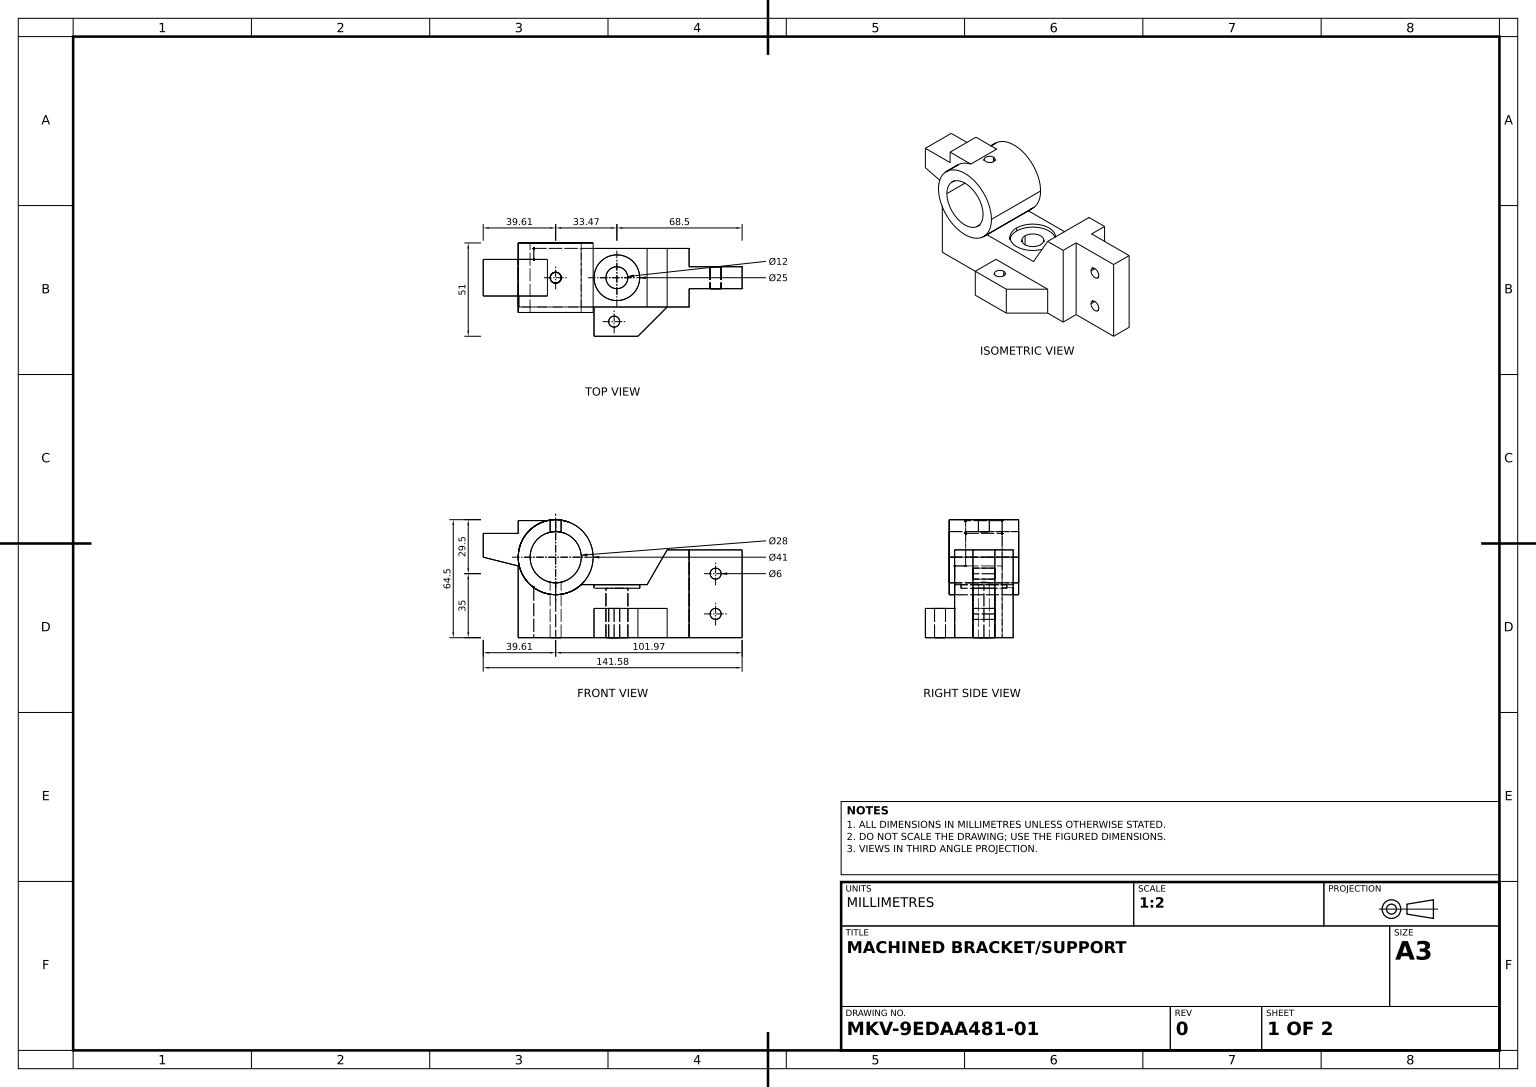
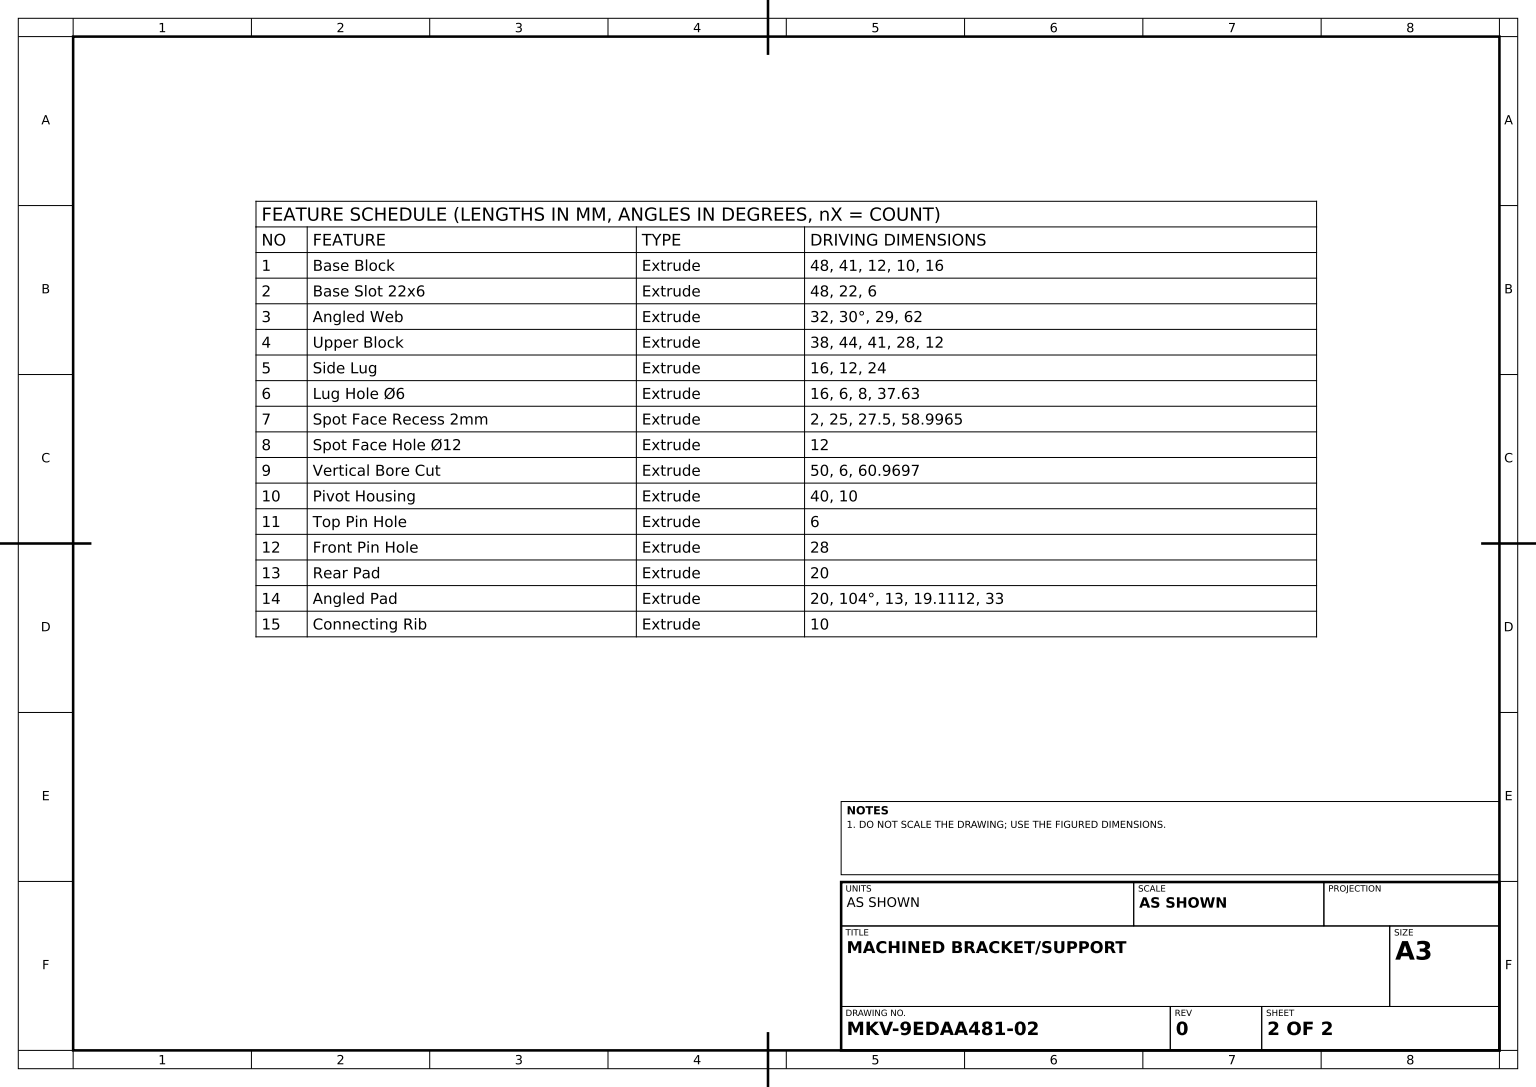
from build123d import *

# Parameters (mm, degrees)
BASE_BLOCK_DEPTH           = 24
BASE_SLOT_SKETCH_R         = 3
BASE_SLOT_22X6_DEPTH       = 48
ANGLED_WEB_DEPTH           = 16
UPPER_BLOCK_SKETCH_R       = 20.5
UPPER_BLOCK_SKETCH_R_2     = 14
UPPER_BLOCK_DEPTH          = 19
SIDE_LUG_SKETCH_W          = 24
SIDE_LUG_SKETCH_H          = 16
SIDE_LUG_DEPTH             = 16
LUG_HOLE_SKETCH_R          = 3
LUG_HOLE_6_DEPTH           = 16
SPOT_FACE_RECESS_SKETCH_R  = 12.5
SPOT_FACE_RECESS_2MM_DEPTH = 2
SPOT_FACE_HOLE_SKETCH_R    = 6
SPOT_FACE_HOLE_12_DEPTH    = 96.223708731
VERTICAL_BORE_SKETCH_R     = 3
VERTICAL_BORE_CUT_DEPTH    = 50
PIVOT_HOUSING_DEPTH        = 40
TOP_PIN_HOLE_DEPTH         = 97.444568168
TOP_PIN_HOLE_DEPTH_BACK    = 97.444568168
TOP_PIN_HOLE_SKETCH_R      = 3
FRONT_PIN_HOLE_DEPTH       = 97.444568168
FRONT_PIN_HOLE_DEPTH_BACK  = 97.444568168
FRONT_PIN_HOLE_SKETCH_R    = 14
REAR_PAD_SKETCH_W          = 8.5
REAR_PAD_SKETCH_H          = 24
REAR_PAD_DEPTH             = 20
ANGLED_PAD_DEPTH           = 10
CONNECTING_RIB_DEPTH       = 10


with BuildPart() as part:
    # Base Block Sketch → Base Block (new, symmetric)
    with BuildSketch(Plane(origin=(0, 0, 0), x_dir=(1, 0, 0), z_dir=(0, 1, 0))):
        Polygon((0, -16), (0, 16), (12, 16), (12, 6), (41, 6), (41, -6), (12, -6), (12, -16), align=None)
    extrude(amount=BASE_BLOCK_DEPTH, both=True)

    # Base Slot Sketch → Base Slot 22x6 (cut)
    with BuildSketch(Plane.XY.offset(6)):
        with Locations((26.5, 11)):
            Circle(BASE_SLOT_SKETCH_R)
        with Locations(Location((26.5, -11, 0), (0, 0, 180))):
            Circle(BASE_SLOT_SKETCH_R)
    extrude(amount=-BASE_SLOT_22X6_DEPTH, mode=Mode.SUBTRACT)

    # Angled Web Sketch → Angled Web (add, symmetric)
    with BuildSketch(Plane.XY):
        Polygon((0, -24), (0, 24), (-10.969655115, 5), (-72.969655115, 5), (-72.969655115, -24), align=None)
    extrude(amount=ANGLED_WEB_DEPTH, both=True)

    # Upper Block Sketch → Upper Block (add, symmetric)
    with BuildSketch(Plane.XY):
        with Locations((-60.969655115, 20)):
            Circle(UPPER_BLOCK_SKETCH_R)
        with Locations((-60.969655115, 20)):
            Circle(UPPER_BLOCK_SKETCH_R_2, mode=Mode.SUBTRACT)
    extrude(amount=UPPER_BLOCK_DEPTH, both=True)

    # Side Lug Sketch → Side Lug (add)
    with BuildSketch(Plane.XZ.offset(24)):
        with Locations((-28, 24)):
            Rectangle(SIDE_LUG_SKETCH_W, SIDE_LUG_SKETCH_H)
        Polygon((-16, 16), (0, 16), (-16, 32), align=None)
    extrude(amount=-SIDE_LUG_DEPTH)

    # Lug Hole Sketch → Lug Hole Ø6 (cut)
    with BuildSketch(Plane(origin=(0, -8, 0), x_dir=(1, 0, 0), z_dir=(0, 1, 0))):
        with Locations(Location((-28.983060808, -24, 0), (0, 0, 270))):
            Circle(LUG_HOLE_SKETCH_R)
    extrude(amount=-LUG_HOLE_6_DEPTH, mode=Mode.SUBTRACT)

    # Spot Face Recess Sketch → Spot Face Recess 2mm (cut)
    with BuildSketch(Plane(origin=(0, 5, 0), x_dir=(1, 0, 0), z_dir=(0, 1, 0))):
        with Locations(Location((-27.5, 0, 0), (0, 0, 180))):
            Circle(SPOT_FACE_RECESS_SKETCH_R)
    extrude(amount=-SPOT_FACE_RECESS_2MM_DEPTH, mode=Mode.SUBTRACT)

    # Spot Face Hole Sketch → Spot Face Hole Ø12 (cut, through all)
    with BuildSketch(Plane(origin=(0, 3, 0), x_dir=(1, 0, 0), z_dir=(0, 1, 0))):
        with Locations(Location((-27.5, 0, 0), (0, 0, 180))):
            Circle(SPOT_FACE_HOLE_SKETCH_R)
    extrude(amount=-SPOT_FACE_HOLE_12_DEPTH, mode=Mode.SUBTRACT)

    # Vertical Bore Sketch → Vertical Bore Cut (cut)
    with BuildSketch(Plane(origin=(0, 0, 0), x_dir=(1, 0, 0), z_dir=(0, 1, 0))):
        with Locations(Location((-60.969655115, 0, 0), (0, 0, 90))):
            Circle(VERTICAL_BORE_SKETCH_R)
    extrude(amount=VERTICAL_BORE_CUT_DEPTH, mode=Mode.SUBTRACT)

    # Pivot Housing Sketch → Pivot Housing (add)
    with BuildSketch(Plane(origin=(0, 0, 0), x_dir=(1, 0, 0), z_dir=(0, 1, 0))):
        Polygon((-60.969655115, 0), (-60.969655115, 10), (-81.469655115, 10), (-81.469655115, -10), (-60.969655115, -10), align=None)
    extrude(amount=PIVOT_HOUSING_DEPTH)

    # Top Pin Hole Sketch → Top Pin Hole (cut, two sides: drawn at the far end of the back side and taken through both)
    with BuildSketch(Plane(origin=(0, 0, 0), x_dir=(1, 0, 0), z_dir=(0, 1, 0)).offset(-TOP_PIN_HOLE_DEPTH_BACK)):
        with Locations(Location((-60.969655115, 0, 0), (0, 0, 90))):
            Circle(TOP_PIN_HOLE_SKETCH_R)
    extrude(amount=TOP_PIN_HOLE_DEPTH + TOP_PIN_HOLE_DEPTH_BACK, mode=Mode.SUBTRACT)

    # Front Pin Hole Sketch → Front Pin Hole (cut, two sides: drawn at the far end of the back side and taken through both)
    with BuildSketch(Plane.XY.offset(-FRONT_PIN_HOLE_DEPTH_BACK)):
        with Locations((-60.969655115, 20)):
            Circle(FRONT_PIN_HOLE_SKETCH_R)
    extrude(amount=FRONT_PIN_HOLE_DEPTH + FRONT_PIN_HOLE_DEPTH_BACK, mode=Mode.SUBTRACT)

    # Rear Pad Sketch → Rear Pad (add)
    with BuildSketch(Plane.XY.offset(10)):
        with Locations((-77.219655115, -12)):
            Rectangle(REAR_PAD_SKETCH_W, REAR_PAD_SKETCH_H)
    extrude(amount=-REAR_PAD_DEPTH)

    # Angled Pad Sketch → Angled Pad (add, symmetric)
    with BuildSketch(Plane.XY):
        Polygon((-100.580876389, 20), (-100.580876389, 33), (-81.469655115, 33), (-81.469655115, 15.235037368), align=None)
    extrude(amount=ANGLED_PAD_DEPTH, both=True)

    # Connecting Rib Sketch → Connecting Rib (add)
    with BuildSketch(Plane.XY.offset(16)):
        with BuildLine():
            Line((-72.969655115, -24), (-81.469655115, -24))
            Line((-81.469655115, -24), (-81.469655115, 15.235037368))
            Line((-81.469655115, 15.235037368), (-80.90818894, 15.235037368))
            ThreePointArc((-80.90818894, 15.235037368), (-78.003666053, 8.594191332), (-72.969655115, 3.379229861))
            Line((-72.969655115, 3.379229861), (-72.969655115, -24))
        make_face()
    extrude(amount=-CONNECTING_RIB_DEPTH)


solid = part.part
